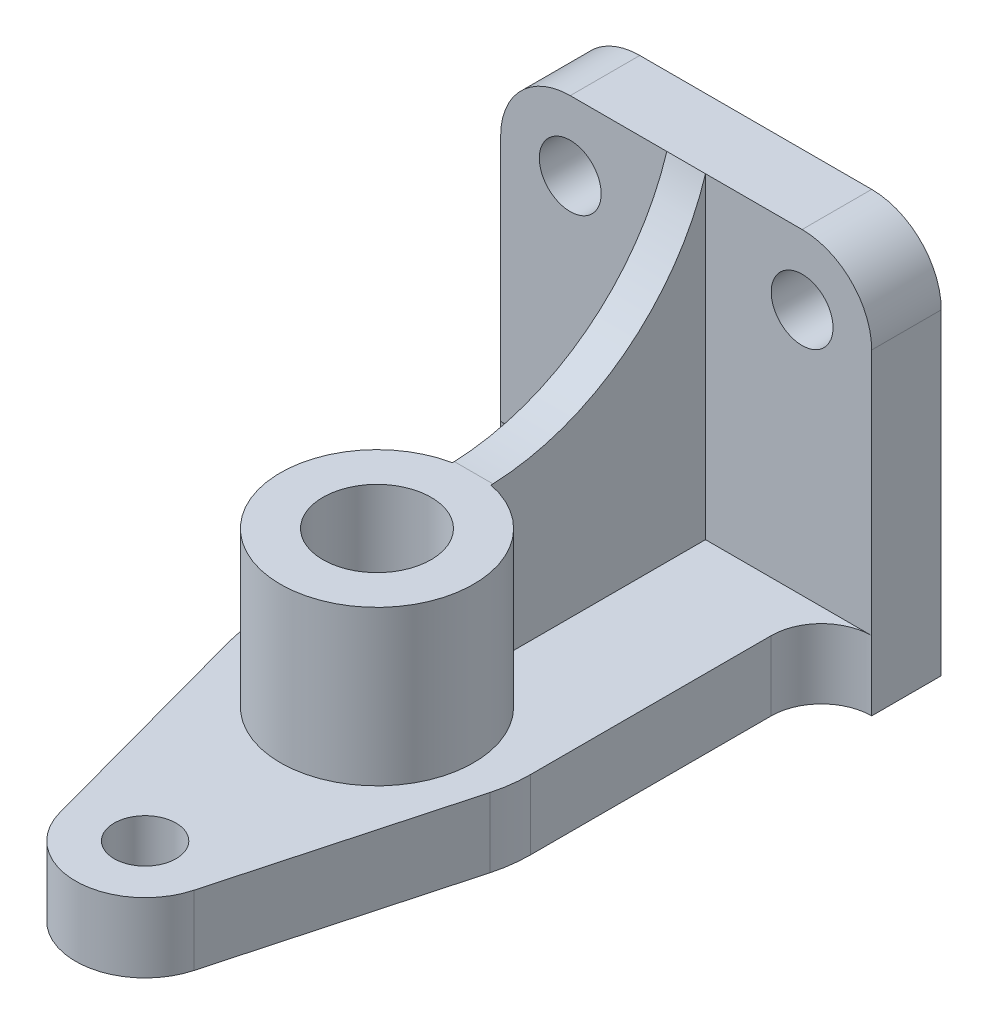
ISO-10303-21;
HEADER;
FILE_DESCRIPTION(('STEP AP214'),'2;1');
FILE_NAME('part.step','',(''),(''),'','','');
FILE_SCHEMA(('AUTOMOTIVE_DESIGN { 1 0 10303 214 1 1 1 1 }'));
ENDSEC;
DATA;
#1=APPLICATION_CONTEXT('core data for automotive mechanical design processes');
#2=APPLICATION_PROTOCOL_DEFINITION('international standard','automotive_design',2000,#1);
#3=PRODUCT_CONTEXT('',#1,'mechanical');
#4=PRODUCT('Part','Part','',(#3));
#5=PRODUCT_RELATED_PRODUCT_CATEGORY('part','',(#4));
#6=PRODUCT_DEFINITION_FORMATION('','',#4);
#7=PRODUCT_DEFINITION_CONTEXT('part definition',#1,'design');
#8=PRODUCT_DEFINITION('design','',#6,#7);
#9=PRODUCT_DEFINITION_SHAPE('','',#8);
#10=(LENGTH_UNIT() NAMED_UNIT(*) SI_UNIT(.MILLI.,.METRE.));
#11=(NAMED_UNIT(*) PLANE_ANGLE_UNIT() SI_UNIT($,.RADIAN.));
#12=(NAMED_UNIT(*) SI_UNIT($,.STERADIAN.) SOLID_ANGLE_UNIT());
#13=UNCERTAINTY_MEASURE_WITH_UNIT(LENGTH_MEASURE(1.E-05),#10,'distance_accuracy_value','');
#14=(GEOMETRIC_REPRESENTATION_CONTEXT(3) GLOBAL_UNCERTAINTY_ASSIGNED_CONTEXT((#13)) GLOBAL_UNIT_ASSIGNED_CONTEXT((#10,
#11,#12)) REPRESENTATION_CONTEXT('',''));
#15=CARTESIAN_POINT('',(0.,0.,0.));
#16=DIRECTION('',(0.,0.,1.));
#17=DIRECTION('',(1.,0.,0.));
#18=AXIS2_PLACEMENT_3D('',#15,#16,#17);
#19=CARTESIAN_POINT('',(18.,82.,18.));
#20=DIRECTION('',(0.,0.,-1.));
#21=DIRECTION('',(-1.,0.,0.));
#22=AXIS2_PLACEMENT_3D('',#19,#20,#21);
#23=PLANE('',#22);
#24=CARTESIAN_POINT('',(18.,82.,18.));
#25=DIRECTION('',(0.,0.,1.));
#26=DIRECTION('',(1.,0.,0.));
#27=AXIS2_PLACEMENT_3D('',#24,#25,#26);
#28=CIRCLE('',#27,8.);
#29=CARTESIAN_POINT('',(26.,82.,18.));
#30=VERTEX_POINT('',#29);
#31=EDGE_CURVE('E290',#30,#30,#28,.T.);
#32=ORIENTED_EDGE('',*,*,#31,.F.);
#33=EDGE_LOOP('',(#32));
#34=FACE_BOUND('',#33,.T.);
#35=DIRECTION('',(0.,-1.,0.));
#36=VECTOR('',#35,1.);
#37=CARTESIAN_POINT('',(43.,82.,18.));
#38=LINE('',#37,#36);
#39=CARTESIAN_POINT('',(43.,100.,18.));
#40=VERTEX_POINT('',#39);
#41=CARTESIAN_POINT('',(43.,18.,18.));
#42=VERTEX_POINT('',#41);
#43=EDGE_CURVE('E209',#40,#42,#38,.T.);
#44=ORIENTED_EDGE('',*,*,#43,.F.);
#45=DIRECTION('',(-1.,0.,0.));
#46=VECTOR('',#45,1.);
#47=CARTESIAN_POINT('',(18.0000000000001,100.,18.));
#48=LINE('',#47,#46);
#49=CARTESIAN_POINT('',(18.0000000000001,100.,18.));
#50=VERTEX_POINT('',#49);
#51=EDGE_CURVE('E303',#40,#50,#48,.T.);
#52=ORIENTED_EDGE('',*,*,#51,.T.);
#53=CARTESIAN_POINT('',(18.,82.,18.));
#54=DIRECTION('',(0.,0.,1.));
#55=DIRECTION('',(-1.,0.,0.));
#56=AXIS2_PLACEMENT_3D('',#53,#54,#55);
#57=CIRCLE('',#56,18.);
#58=CARTESIAN_POINT('',(0.,81.9999999999999,18.));
#59=VERTEX_POINT('',#58);
#60=EDGE_CURVE('E310',#50,#59,#57,.T.);
#61=ORIENTED_EDGE('',*,*,#60,.T.);
#62=DIRECTION('',(0.,-1.,0.));
#63=VECTOR('',#62,1.);
#64=CARTESIAN_POINT('',(0.,0.,18.));
#65=LINE('',#64,#63);
#66=CARTESIAN_POINT('',(0.,18.,18.));
#67=VERTEX_POINT('',#66);
#68=EDGE_CURVE('E291',#59,#67,#65,.T.);
#69=ORIENTED_EDGE('',*,*,#68,.T.);
#70=DIRECTION('',(1.,0.,0.));
#71=VECTOR('',#70,1.);
#72=CARTESIAN_POINT('',(13.,18.,18.));
#73=LINE('',#72,#71);
#74=EDGE_CURVE('E279',#67,#42,#73,.T.);
#75=ORIENTED_EDGE('',*,*,#74,.T.);
#76=EDGE_LOOP('',(#44,#52,#61,#69,#75));
#77=FACE_BOUND('',#76,.T.);
#78=ADVANCED_FACE('F45',(#34,#77),#23,.F.);
#79=CARTESIAN_POINT('',(0.,0.,18.));
#80=DIRECTION('',(0.,1.,0.));
#81=DIRECTION('',(0.,0.,1.));
#82=AXIS2_PLACEMENT_3D('',#79,#80,#81);
#83=PLANE('',#82);
#84=CARTESIAN_POINT('',(48.,0.,158.));
#85=DIRECTION('',(0.,1.,0.));
#86=DIRECTION('',(0.,0.,1.));
#87=AXIS2_PLACEMENT_3D('',#84,#85,#86);
#88=CIRCLE('',#87,8.);
#89=CARTESIAN_POINT('',(48.,0.,166.));
#90=VERTEX_POINT('',#89);
#91=EDGE_CURVE('E217',#90,#90,#88,.T.);
#92=ORIENTED_EDGE('',*,*,#91,.T.);
#93=EDGE_LOOP('',(#92));
#94=FACE_BOUND('',#93,.T.);
#95=DIRECTION('',(-0.262825333985644,0.,0.964843429689675));
#96=VECTOR('',#95,1.);
#97=CARTESIAN_POINT('',(97.5534197688363,0.,44.5737521168928));
#98=LINE('',#97,#96);
#99=CARTESIAN_POINT('',(81.7695200391386,0.,102.517146378541));
#100=VERTEX_POINT('',#99);
#101=CARTESIAN_POINT('',(65.3671817344141,0.,162.730856011742));
#102=VERTEX_POINT('',#101);
#103=EDGE_CURVE('E251',#100,#102,#98,.T.);
#104=ORIENTED_EDGE('',*,*,#103,.T.);
#105=CARTESIAN_POINT('',(48.,0.,158.));
#106=DIRECTION('',(0.,1.,0.));
#107=DIRECTION('',(0.,0.,1.));
#108=AXIS2_PLACEMENT_3D('',#105,#106,#107);
#109=CIRCLE('',#108,18.);
#110=CARTESIAN_POINT('',(30.6328182655859,0.,162.730856011742));
#111=VERTEX_POINT('',#110);
#112=EDGE_CURVE('E228',#111,#102,#109,.T.);
#113=ORIENTED_EDGE('',*,*,#112,.F.);
#114=DIRECTION('',(0.262825333985644,0.,0.964843429689675));
#115=VECTOR('',#114,1.);
#116=CARTESIAN_POINT('',(-8.18482676256409,0.,20.2295636382967));
#117=LINE('',#116,#115);
#118=CARTESIAN_POINT('',(14.2304799608614,0.,102.51714637854));
#119=VERTEX_POINT('',#118);
#120=EDGE_CURVE('E260',#119,#111,#117,.T.);
#121=ORIENTED_EDGE('',*,*,#120,.F.);
#122=CARTESIAN_POINT('',(48.,0.,93.3182596890428));
#123=DIRECTION('',(0.,1.,0.));
#124=DIRECTION('',(0.,0.,1.));
#125=AXIS2_PLACEMENT_3D('',#122,#123,#124);
#126=CIRCLE('',#125,35.);
#127=CARTESIAN_POINT('',(13.,0.,93.3182596890427));
#128=VERTEX_POINT('',#127);
#129=EDGE_CURVE('E255',#128,#119,#126,.T.);
#130=ORIENTED_EDGE('',*,*,#129,.F.);
#131=DIRECTION('',(0.,0.,-1.));
#132=VECTOR('',#131,1.);
#133=CARTESIAN_POINT('',(13.,0.,18.));
#134=LINE('',#133,#132);
#135=CARTESIAN_POINT('',(13.,0.,31.));
#136=VERTEX_POINT('',#135);
#137=EDGE_CURVE('E272',#128,#136,#134,.T.);
#138=ORIENTED_EDGE('',*,*,#137,.T.);
#139=CARTESIAN_POINT('',(0.,0.,31.));
#140=DIRECTION('',(0.,1.,0.));
#141=DIRECTION('',(0.,0.,1.));
#142=AXIS2_PLACEMENT_3D('',#139,#140,#141);
#143=CIRCLE('',#142,13.);
#144=CARTESIAN_POINT('',(0.,0.,18.));
#145=VERTEX_POINT('',#144);
#146=EDGE_CURVE('E346',#136,#145,#143,.T.);
#147=ORIENTED_EDGE('',*,*,#146,.T.);
#148=DIRECTION('',(0.,0.,-1.));
#149=VECTOR('',#148,1.);
#150=CARTESIAN_POINT('',(0.,0.,18.));
#151=LINE('',#150,#149);
#152=CARTESIAN_POINT('',(0.,0.,0.));
#153=VERTEX_POINT('',#152);
#154=EDGE_CURVE('E337',#145,#153,#151,.T.);
#155=ORIENTED_EDGE('',*,*,#154,.T.);
#156=DIRECTION('',(1.,0.,0.));
#157=VECTOR('',#156,1.);
#158=CARTESIAN_POINT('',(0.,0.,0.));
#159=LINE('',#158,#157);
#160=CARTESIAN_POINT('',(96.,0.,0.));
#161=VERTEX_POINT('',#160);
#162=EDGE_CURVE('E315',#153,#161,#159,.T.);
#163=ORIENTED_EDGE('',*,*,#162,.T.);
#164=DIRECTION('',(0.,0.,-1.));
#165=VECTOR('',#164,1.);
#166=CARTESIAN_POINT('',(96.,0.,18.));
#167=LINE('',#166,#165);
#168=CARTESIAN_POINT('',(96.,0.,18.));
#169=VERTEX_POINT('',#168);
#170=EDGE_CURVE('E331',#169,#161,#167,.T.);
#171=ORIENTED_EDGE('',*,*,#170,.F.);
#172=CARTESIAN_POINT('',(96.,0.,31.));
#173=DIRECTION('',(0.,1.,0.));
#174=DIRECTION('',(0.,0.,1.));
#175=AXIS2_PLACEMENT_3D('',#172,#173,#174);
#176=CIRCLE('',#175,13.);
#177=CARTESIAN_POINT('',(83.,0.,31.));
#178=VERTEX_POINT('',#177);
#179=EDGE_CURVE('E355',#169,#178,#176,.T.);
#180=ORIENTED_EDGE('',*,*,#179,.T.);
#181=DIRECTION('',(0.,0.,-1.));
#182=VECTOR('',#181,1.);
#183=CARTESIAN_POINT('',(83.,0.,18.));
#184=LINE('',#183,#182);
#185=CARTESIAN_POINT('',(83.,0.,93.318259689043));
#186=VERTEX_POINT('',#185);
#187=EDGE_CURVE('E275',#186,#178,#184,.T.);
#188=ORIENTED_EDGE('',*,*,#187,.F.);
#189=CARTESIAN_POINT('',(48.,0.,93.318259689043));
#190=DIRECTION('',(0.,1.,0.));
#191=DIRECTION('',(0.,0.,1.));
#192=AXIS2_PLACEMENT_3D('',#189,#190,#191);
#193=CIRCLE('',#192,35.);
#194=EDGE_CURVE('E242',#100,#186,#193,.T.);
#195=ORIENTED_EDGE('',*,*,#194,.F.);
#196=EDGE_LOOP('',(#104,#113,#121,#130,#138,#147,#155,#163,#171,#180,#188,#195));
#197=FACE_BOUND('',#196,.T.);
#198=ADVANCED_FACE('F417',(#94,#197),#83,.F.);
#199=CARTESIAN_POINT('',(13.,18.,18.));
#200=DIRECTION('',(0.,1.,0.));
#201=DIRECTION('',(0.,0.,1.));
#202=AXIS2_PLACEMENT_3D('',#199,#200,#201);
#203=PLANE('',#202);
#204=CARTESIAN_POINT('',(48.,18.,158.));
#205=DIRECTION('',(0.,1.,0.));
#206=DIRECTION('',(0.,0.,1.));
#207=AXIS2_PLACEMENT_3D('',#204,#205,#206);
#208=CIRCLE('',#207,8.);
#209=CARTESIAN_POINT('',(48.,18.,166.));
#210=VERTEX_POINT('',#209);
#211=EDGE_CURVE('E218',#210,#210,#208,.T.);
#212=ORIENTED_EDGE('',*,*,#211,.F.);
#213=EDGE_LOOP('',(#212));
#214=FACE_BOUND('',#213,.T.);
#215=CARTESIAN_POINT('',(48.,18.,158.));
#216=DIRECTION('',(0.,1.,0.));
#217=DIRECTION('',(0.,0.,1.));
#218=AXIS2_PLACEMENT_3D('',#215,#216,#217);
#219=CIRCLE('',#218,18.);
#220=CARTESIAN_POINT('',(30.6328182655859,18.,162.730856011742));
#221=VERTEX_POINT('',#220);
#222=CARTESIAN_POINT('',(65.3671817344141,18.,162.730856011742));
#223=VERTEX_POINT('',#222);
#224=EDGE_CURVE('E221',#221,#223,#219,.T.);
#225=ORIENTED_EDGE('',*,*,#224,.T.);
#226=DIRECTION('',(-0.262825333985644,0.,0.964843429689675));
#227=VECTOR('',#226,1.);
#228=CARTESIAN_POINT('',(102.117955108573,18.,27.8171409282168));
#229=LINE('',#228,#227);
#230=CARTESIAN_POINT('',(81.7695200391386,18.,102.517146378541));
#231=VERTEX_POINT('',#230);
#232=EDGE_CURVE('E250',#231,#223,#229,.T.);
#233=ORIENTED_EDGE('',*,*,#232,.F.);
#234=CARTESIAN_POINT('',(48.,18.,93.318259689043));
#235=DIRECTION('',(0.,1.,0.));
#236=DIRECTION('',(0.,0.,1.));
#237=AXIS2_PLACEMENT_3D('',#234,#235,#236);
#238=CIRCLE('',#237,35.);
#239=CARTESIAN_POINT('',(83.,18.,93.3182596890429));
#240=VERTEX_POINT('',#239);
#241=EDGE_CURVE('E231',#231,#240,#238,.T.);
#242=ORIENTED_EDGE('',*,*,#241,.T.);
#243=DIRECTION('',(0.,0.,1.));
#244=VECTOR('',#243,1.);
#245=CARTESIAN_POINT('',(83.,18.,18.));
#246=LINE('',#245,#244);
#247=CARTESIAN_POINT('',(83.,18.,31.));
#248=VERTEX_POINT('',#247);
#249=EDGE_CURVE('E262',#248,#240,#246,.T.);
#250=ORIENTED_EDGE('',*,*,#249,.F.);
#251=CARTESIAN_POINT('',(96.,18.,31.));
#252=DIRECTION('',(0.,1.,0.));
#253=DIRECTION('',(0.,0.,1.));
#254=AXIS2_PLACEMENT_3D('',#251,#252,#253);
#255=CIRCLE('',#254,13.);
#256=CARTESIAN_POINT('',(96.,18.,18.));
#257=VERTEX_POINT('',#256);
#258=EDGE_CURVE('E348',#248,#257,#255,.F.);
#259=ORIENTED_EDGE('',*,*,#258,.T.);
#260=CARTESIAN_POINT('',(53.,18.,18.));
#261=VERTEX_POINT('',#260);
#262=EDGE_CURVE('E274',#261,#257,#73,.T.);
#263=ORIENTED_EDGE('',*,*,#262,.F.);
#264=DIRECTION('',(0.,0.,-1.));
#265=VECTOR('',#264,1.);
#266=CARTESIAN_POINT('',(53.,18.,18.));
#267=LINE('',#266,#265);
#268=CARTESIAN_POINT('',(53.,18.,73.5051025721682));
#269=VERTEX_POINT('',#268);
#270=EDGE_CURVE('E60',#269,#261,#267,.T.);
#271=ORIENTED_EDGE('',*,*,#270,.F.);
#272=CARTESIAN_POINT('',(48.,18.,98.));
#273=DIRECTION('',(0.,1.,0.));
#274=DIRECTION('',(0.,0.,1.));
#275=AXIS2_PLACEMENT_3D('',#272,#273,#274);
#276=CIRCLE('',#275,25.);
#277=CARTESIAN_POINT('',(43.,18.,73.5051025721682));
#278=VERTEX_POINT('',#277);
#279=EDGE_CURVE('E256',#278,#269,#276,.T.);
#280=ORIENTED_EDGE('',*,*,#279,.F.);
#281=DIRECTION('',(0.,0.,-1.));
#282=VECTOR('',#281,1.);
#283=CARTESIAN_POINT('',(43.,18.,18.));
#284=LINE('',#283,#282);
#285=EDGE_CURVE('E63',#278,#42,#284,.T.);
#286=ORIENTED_EDGE('',*,*,#285,.T.);
#287=ORIENTED_EDGE('',*,*,#74,.F.);
#288=CARTESIAN_POINT('',(0.,18.,31.));
#289=DIRECTION('',(0.,1.,0.));
#290=DIRECTION('',(0.,0.,1.));
#291=AXIS2_PLACEMENT_3D('',#288,#289,#290);
#292=CIRCLE('',#291,13.);
#293=CARTESIAN_POINT('',(13.,18.,31.));
#294=VERTEX_POINT('',#293);
#295=EDGE_CURVE('E343',#67,#294,#292,.F.);
#296=ORIENTED_EDGE('',*,*,#295,.T.);
#297=DIRECTION('',(0.,0.,1.));
#298=VECTOR('',#297,1.);
#299=CARTESIAN_POINT('',(13.,18.,18.));
#300=LINE('',#299,#298);
#301=CARTESIAN_POINT('',(13.,18.,93.3182596890427));
#302=VERTEX_POINT('',#301);
#303=EDGE_CURVE('E266',#294,#302,#300,.T.);
#304=ORIENTED_EDGE('',*,*,#303,.T.);
#305=CARTESIAN_POINT('',(48.,18.,93.3182596890428));
#306=DIRECTION('',(0.,1.,0.));
#307=DIRECTION('',(0.,0.,1.));
#308=AXIS2_PLACEMENT_3D('',#305,#306,#307);
#309=CIRCLE('',#308,35.);
#310=CARTESIAN_POINT('',(14.2304799608614,18.,102.51714637854));
#311=VERTEX_POINT('',#310);
#312=EDGE_CURVE('E236',#302,#311,#309,.T.);
#313=ORIENTED_EDGE('',*,*,#312,.T.);
#314=DIRECTION('',(0.262825333985644,0.,0.964843429689675));
#315=VECTOR('',#314,1.);
#316=CARTESIAN_POINT('',(-12.7493621023009,18.,3.47295244962065));
#317=LINE('',#316,#315);
#318=EDGE_CURVE('E237',#311,#221,#317,.T.);
#319=ORIENTED_EDGE('',*,*,#318,.T.);
#320=EDGE_LOOP('',(#225,#233,#242,#250,#259,#263,#271,#280,#286,#287,#296,#304,#313,#319));
#321=FACE_BOUND('',#320,.T.);
#322=ADVANCED_FACE('F370',(#214,#321),#203,.T.);
#323=CARTESIAN_POINT('',(78.,82.,18.));
#324=DIRECTION('',(0.,0.,1.));
#325=DIRECTION('',(1.,0.,0.));
#326=AXIS2_PLACEMENT_3D('',#323,#324,#325);
#327=CIRCLE('',#326,8.00000000000001);
#328=CARTESIAN_POINT('',(86.,82.,18.));
#329=VERTEX_POINT('',#328);
#330=EDGE_CURVE('E284',#329,#329,#327,.T.);
#331=ORIENTED_EDGE('',*,*,#330,.F.);
#332=EDGE_LOOP('',(#331));
#333=FACE_BOUND('',#332,.T.);
#334=CARTESIAN_POINT('',(77.9999999999999,100.,18.));
#335=VERTEX_POINT('',#334);
#336=CARTESIAN_POINT('',(53.,100.,18.));
#337=VERTEX_POINT('',#336);
#338=EDGE_CURVE('E302',#335,#337,#48,.T.);
#339=ORIENTED_EDGE('',*,*,#338,.T.);
#340=DIRECTION('',(0.,-1.,0.));
#341=VECTOR('',#340,1.);
#342=CARTESIAN_POINT('',(53.,82.,18.));
#343=LINE('',#342,#341);
#344=EDGE_CURVE('E211',#337,#261,#343,.T.);
#345=ORIENTED_EDGE('',*,*,#344,.T.);
#346=ORIENTED_EDGE('',*,*,#262,.T.);
#347=DIRECTION('',(0.,1.,0.));
#348=VECTOR('',#347,1.);
#349=CARTESIAN_POINT('',(96.,0.,18.));
#350=LINE('',#349,#348);
#351=CARTESIAN_POINT('',(96.,81.9999999999999,18.));
#352=VERTEX_POINT('',#351);
#353=EDGE_CURVE('E298',#257,#352,#350,.T.);
#354=ORIENTED_EDGE('',*,*,#353,.T.);
#355=CARTESIAN_POINT('',(78.,82.,18.));
#356=DIRECTION('',(0.,0.,1.));
#357=DIRECTION('',(-1.,0.,0.));
#358=AXIS2_PLACEMENT_3D('',#355,#356,#357);
#359=CIRCLE('',#358,18.);
#360=EDGE_CURVE('E301',#352,#335,#359,.T.);
#361=ORIENTED_EDGE('',*,*,#360,.T.);
#362=EDGE_LOOP('',(#339,#345,#346,#354,#361));
#363=FACE_BOUND('',#362,.T.);
#364=ADVANCED_FACE('F379',(#333,#363),#23,.F.);
#365=CARTESIAN_POINT('',(18.,82.,0.));
#366=DIRECTION('',(0.,0.,-1.));
#367=DIRECTION('',(-1.,0.,0.));
#368=AXIS2_PLACEMENT_3D('',#365,#366,#367);
#369=PLANE('',#368);
#370=DIRECTION('',(0.,1.,0.));
#371=VECTOR('',#370,1.);
#372=CARTESIAN_POINT('',(96.,0.,0.));
#373=LINE('',#372,#371);
#374=CARTESIAN_POINT('',(96.,81.9999999999999,0.));
#375=VERTEX_POINT('',#374);
#376=EDGE_CURVE('E313',#161,#375,#373,.T.);
#377=ORIENTED_EDGE('',*,*,#376,.F.);
#378=ORIENTED_EDGE('',*,*,#162,.F.);
#379=DIRECTION('',(0.,-1.,0.));
#380=VECTOR('',#379,1.);
#381=CARTESIAN_POINT('',(0.,0.,0.));
#382=LINE('',#381,#380);
#383=CARTESIAN_POINT('',(0.,81.9999999999999,0.));
#384=VERTEX_POINT('',#383);
#385=EDGE_CURVE('E287',#384,#153,#382,.T.);
#386=ORIENTED_EDGE('',*,*,#385,.F.);
#387=CARTESIAN_POINT('',(18.,82.,0.));
#388=DIRECTION('',(0.,0.,1.));
#389=DIRECTION('',(-1.,0.,0.));
#390=AXIS2_PLACEMENT_3D('',#387,#388,#389);
#391=CIRCLE('',#390,18.);
#392=CARTESIAN_POINT('',(18.0000000000001,100.,0.));
#393=VERTEX_POINT('',#392);
#394=EDGE_CURVE('E318',#393,#384,#391,.T.);
#395=ORIENTED_EDGE('',*,*,#394,.F.);
#396=DIRECTION('',(-1.,0.,0.));
#397=VECTOR('',#396,1.);
#398=CARTESIAN_POINT('',(18.0000000000001,100.,0.));
#399=LINE('',#398,#397);
#400=CARTESIAN_POINT('',(77.9999999999999,100.,0.));
#401=VERTEX_POINT('',#400);
#402=EDGE_CURVE('E319',#401,#393,#399,.T.);
#403=ORIENTED_EDGE('',*,*,#402,.F.);
#404=CARTESIAN_POINT('',(78.,82.,0.));
#405=DIRECTION('',(0.,0.,1.));
#406=DIRECTION('',(-1.,0.,0.));
#407=AXIS2_PLACEMENT_3D('',#404,#405,#406);
#408=CIRCLE('',#407,18.);
#409=EDGE_CURVE('E317',#375,#401,#408,.T.);
#410=ORIENTED_EDGE('',*,*,#409,.F.);
#411=EDGE_LOOP('',(#377,#378,#386,#395,#403,#410));
#412=FACE_BOUND('',#411,.T.);
#413=CARTESIAN_POINT('',(78.,82.,0.));
#414=DIRECTION('',(0.,0.,1.));
#415=DIRECTION('',(1.,0.,0.));
#416=AXIS2_PLACEMENT_3D('',#413,#414,#415);
#417=CIRCLE('',#416,8.00000000000001);
#418=CARTESIAN_POINT('',(86.,82.,0.));
#419=VERTEX_POINT('',#418);
#420=EDGE_CURVE('E278',#419,#419,#417,.T.);
#421=ORIENTED_EDGE('',*,*,#420,.T.);
#422=EDGE_LOOP('',(#421));
#423=FACE_BOUND('',#422,.T.);
#424=CARTESIAN_POINT('',(18.,82.,0.));
#425=DIRECTION('',(0.,0.,1.));
#426=DIRECTION('',(1.,0.,0.));
#427=AXIS2_PLACEMENT_3D('',#424,#425,#426);
#428=CIRCLE('',#427,8.);
#429=CARTESIAN_POINT('',(26.,82.,0.));
#430=VERTEX_POINT('',#429);
#431=EDGE_CURVE('E283',#430,#430,#428,.T.);
#432=ORIENTED_EDGE('',*,*,#431,.T.);
#433=EDGE_LOOP('',(#432));
#434=FACE_BOUND('',#433,.T.);
#435=ADVANCED_FACE('F434',(#412,#423,#434),#369,.T.);
#436=CARTESIAN_POINT('',(0.,0.,18.));
#437=DIRECTION('',(1.,0.,0.));
#438=DIRECTION('',(0.,0.,-1.));
#439=AXIS2_PLACEMENT_3D('',#436,#437,#438);
#440=PLANE('',#439);
#441=ORIENTED_EDGE('',*,*,#385,.T.);
#442=ORIENTED_EDGE('',*,*,#154,.F.);
#443=EDGE_CURVE('E300',#67,#145,#65,.T.);
#444=ORIENTED_EDGE('',*,*,#443,.F.);
#445=ORIENTED_EDGE('',*,*,#68,.F.);
#446=DIRECTION('',(0.,0.,-1.));
#447=VECTOR('',#446,1.);
#448=CARTESIAN_POINT('',(0.,81.9999999999999,18.));
#449=LINE('',#448,#447);
#450=EDGE_CURVE('E307',#59,#384,#449,.T.);
#451=ORIENTED_EDGE('',*,*,#450,.T.);
#452=EDGE_LOOP('',(#441,#442,#444,#445,#451));
#453=FACE_BOUND('',#452,.T.);
#454=ADVANCED_FACE('F402',(#453),#440,.F.);
#455=CARTESIAN_POINT('',(96.,0.,18.));
#456=DIRECTION('',(-1.,0.,0.));
#457=DIRECTION('',(0.,0.,1.));
#458=AXIS2_PLACEMENT_3D('',#455,#456,#457);
#459=PLANE('',#458);
#460=ORIENTED_EDGE('',*,*,#376,.T.);
#461=DIRECTION('',(0.,0.,-1.));
#462=VECTOR('',#461,1.);
#463=CARTESIAN_POINT('',(96.,81.9999999999999,18.));
#464=LINE('',#463,#462);
#465=EDGE_CURVE('E327',#352,#375,#464,.T.);
#466=ORIENTED_EDGE('',*,*,#465,.F.);
#467=ORIENTED_EDGE('',*,*,#353,.F.);
#468=EDGE_CURVE('E296',#169,#257,#350,.T.);
#469=ORIENTED_EDGE('',*,*,#468,.F.);
#470=ORIENTED_EDGE('',*,*,#170,.T.);
#471=EDGE_LOOP('',(#460,#466,#467,#469,#470));
#472=FACE_BOUND('',#471,.T.);
#473=ADVANCED_FACE('F380',(#472),#459,.F.);
#474=CARTESIAN_POINT('',(78.,82.,18.));
#475=DIRECTION('',(0.,0.,-1.));
#476=DIRECTION('',(-1.,0.,0.));
#477=AXIS2_PLACEMENT_3D('',#474,#475,#476);
#478=CYLINDRICAL_SURFACE('',#477,18.);
#479=ORIENTED_EDGE('',*,*,#409,.T.);
#480=DIRECTION('',(0.,0.,-1.));
#481=VECTOR('',#480,1.);
#482=CARTESIAN_POINT('',(77.9999999999999,100.,18.));
#483=LINE('',#482,#481);
#484=EDGE_CURVE('E326',#335,#401,#483,.T.);
#485=ORIENTED_EDGE('',*,*,#484,.F.);
#486=ORIENTED_EDGE('',*,*,#360,.F.);
#487=ORIENTED_EDGE('',*,*,#465,.T.);
#488=EDGE_LOOP('',(#479,#485,#486,#487));
#489=FACE_BOUND('',#488,.T.);
#490=ADVANCED_FACE('F438',(#489),#478,.T.);
#491=CARTESIAN_POINT('',(18.0000000000001,100.,18.));
#492=DIRECTION('',(0.,-1.,0.));
#493=DIRECTION('',(0.,0.,-1.));
#494=AXIS2_PLACEMENT_3D('',#491,#492,#493);
#495=PLANE('',#494);
#496=ORIENTED_EDGE('',*,*,#402,.T.);
#497=DIRECTION('',(0.,0.,-1.));
#498=VECTOR('',#497,1.);
#499=CARTESIAN_POINT('',(18.0000000000001,100.,18.));
#500=LINE('',#499,#498);
#501=EDGE_CURVE('E321',#50,#393,#500,.T.);
#502=ORIENTED_EDGE('',*,*,#501,.F.);
#503=ORIENTED_EDGE('',*,*,#51,.F.);
#504=DIRECTION('',(1.,0.,0.));
#505=VECTOR('',#504,1.);
#506=CARTESIAN_POINT('',(48.,100.,18.));
#507=LINE('',#506,#505);
#508=EDGE_CURVE('E194',#40,#337,#507,.T.);
#509=ORIENTED_EDGE('',*,*,#508,.T.);
#510=ORIENTED_EDGE('',*,*,#338,.F.);
#511=ORIENTED_EDGE('',*,*,#484,.T.);
#512=EDGE_LOOP('',(#496,#502,#503,#509,#510,#511));
#513=FACE_BOUND('',#512,.T.);
#514=ADVANCED_FACE('F394',(#513),#495,.F.);
#515=CARTESIAN_POINT('',(18.,82.,18.));
#516=DIRECTION('',(0.,0.,-1.));
#517=DIRECTION('',(-1.,0.,0.));
#518=AXIS2_PLACEMENT_3D('',#515,#516,#517);
#519=CYLINDRICAL_SURFACE('',#518,18.);
#520=ORIENTED_EDGE('',*,*,#394,.T.);
#521=ORIENTED_EDGE('',*,*,#450,.F.);
#522=ORIENTED_EDGE('',*,*,#60,.F.);
#523=ORIENTED_EDGE('',*,*,#501,.T.);
#524=EDGE_LOOP('',(#520,#521,#522,#523));
#525=FACE_BOUND('',#524,.T.);
#526=ADVANCED_FACE('F400',(#525),#519,.T.);
#527=CARTESIAN_POINT('',(18.,82.,18.));
#528=DIRECTION('',(0.,0.,-1.));
#529=DIRECTION('',(-1.,0.,0.));
#530=AXIS2_PLACEMENT_3D('',#527,#528,#529);
#531=CYLINDRICAL_SURFACE('',#530,8.);
#532=ORIENTED_EDGE('',*,*,#31,.T.);
#533=EDGE_LOOP('',(#532));
#534=FACE_BOUND('',#533,.T.);
#535=ORIENTED_EDGE('',*,*,#431,.F.);
#536=EDGE_LOOP('',(#535));
#537=FACE_BOUND('',#536,.T.);
#538=ADVANCED_FACE('F471',(#534,#537),#531,.F.);
#539=CARTESIAN_POINT('',(78.,82.,18.));
#540=DIRECTION('',(0.,0.,-1.));
#541=DIRECTION('',(-1.,0.,0.));
#542=AXIS2_PLACEMENT_3D('',#539,#540,#541);
#543=CYLINDRICAL_SURFACE('',#542,8.00000000000001);
#544=ORIENTED_EDGE('',*,*,#330,.T.);
#545=EDGE_LOOP('',(#544));
#546=FACE_BOUND('',#545,.T.);
#547=ORIENTED_EDGE('',*,*,#420,.F.);
#548=EDGE_LOOP('',(#547));
#549=FACE_BOUND('',#548,.T.);
#550=ADVANCED_FACE('F472',(#546,#549),#543,.F.);
#551=CARTESIAN_POINT('',(13.,0.,0.));
#552=DIRECTION('',(1.,0.,0.));
#553=DIRECTION('',(0.,0.,-1.));
#554=AXIS2_PLACEMENT_3D('',#551,#552,#553);
#555=PLANE('',#554);
#556=ORIENTED_EDGE('',*,*,#137,.F.);
#557=DIRECTION('',(0.,1.,0.));
#558=VECTOR('',#557,1.);
#559=CARTESIAN_POINT('',(13.,-22.,93.3182596890428));
#560=LINE('',#559,#558);
#561=EDGE_CURVE('E12',#128,#302,#560,.T.);
#562=ORIENTED_EDGE('',*,*,#561,.T.);
#563=ORIENTED_EDGE('',*,*,#303,.F.);
#564=DIRECTION('',(0.,1.,0.));
#565=VECTOR('',#564,1.);
#566=CARTESIAN_POINT('',(13.,0.,31.));
#567=LINE('',#566,#565);
#568=EDGE_CURVE('E339',#294,#136,#567,.F.);
#569=ORIENTED_EDGE('',*,*,#568,.T.);
#570=EDGE_LOOP('',(#556,#562,#563,#569));
#571=FACE_BOUND('',#570,.T.);
#572=ADVANCED_FACE('F415',(#571),#555,.F.);
#573=CARTESIAN_POINT('',(83.,0.,0.));
#574=DIRECTION('',(1.,0.,0.));
#575=DIRECTION('',(0.,0.,-1.));
#576=AXIS2_PLACEMENT_3D('',#573,#574,#575);
#577=PLANE('',#576);
#578=DIRECTION('',(0.,1.,0.));
#579=VECTOR('',#578,1.);
#580=CARTESIAN_POINT('',(83.,-22.,93.318259689043));
#581=LINE('',#580,#579);
#582=EDGE_CURVE('E49',#186,#240,#581,.T.);
#583=ORIENTED_EDGE('',*,*,#582,.F.);
#584=ORIENTED_EDGE('',*,*,#187,.T.);
#585=DIRECTION('',(0.,1.,0.));
#586=VECTOR('',#585,1.);
#587=CARTESIAN_POINT('',(83.,0.,31.));
#588=LINE('',#587,#586);
#589=EDGE_CURVE('E345',#178,#248,#588,.T.);
#590=ORIENTED_EDGE('',*,*,#589,.T.);
#591=ORIENTED_EDGE('',*,*,#249,.T.);
#592=EDGE_LOOP('',(#583,#584,#590,#591));
#593=FACE_BOUND('',#592,.T.);
#594=ADVANCED_FACE('F368',(#593),#577,.T.);
#595=CARTESIAN_POINT('',(0.,82.,31.));
#596=DIRECTION('',(0.,-1.,0.));
#597=DIRECTION('',(0.,0.,-1.));
#598=AXIS2_PLACEMENT_3D('',#595,#596,#597);
#599=CYLINDRICAL_SURFACE('',#598,13.);
#600=ORIENTED_EDGE('',*,*,#146,.F.);
#601=ORIENTED_EDGE('',*,*,#568,.F.);
#602=ORIENTED_EDGE('',*,*,#295,.F.);
#603=ORIENTED_EDGE('',*,*,#443,.T.);
#604=EDGE_LOOP('',(#600,#601,#602,#603));
#605=FACE_BOUND('',#604,.T.);
#606=ADVANCED_FACE('F409',(#605),#599,.F.);
#607=CARTESIAN_POINT('',(96.,0.,31.));
#608=DIRECTION('',(0.,1.,0.));
#609=DIRECTION('',(0.,0.,1.));
#610=AXIS2_PLACEMENT_3D('',#607,#608,#609);
#611=CYLINDRICAL_SURFACE('',#610,13.);
#612=ORIENTED_EDGE('',*,*,#179,.F.);
#613=ORIENTED_EDGE('',*,*,#468,.T.);
#614=ORIENTED_EDGE('',*,*,#258,.F.);
#615=ORIENTED_EDGE('',*,*,#589,.F.);
#616=EDGE_LOOP('',(#612,#613,#614,#615));
#617=FACE_BOUND('',#616,.T.);
#618=ADVANCED_FACE('F42',(#617),#611,.F.);
#619=CARTESIAN_POINT('',(48.,58.,98.));
#620=DIRECTION('',(0.,-1.,0.));
#621=DIRECTION('',(0.,0.,-1.));
#622=AXIS2_PLACEMENT_3D('',#619,#620,#621);
#623=CYLINDRICAL_SURFACE('',#622,14.);
#624=CARTESIAN_POINT('',(48.,18.,98.));
#625=DIRECTION('',(0.,1.,0.));
#626=DIRECTION('',(0.,0.,1.));
#627=AXIS2_PLACEMENT_3D('',#624,#625,#626);
#628=CIRCLE('',#627,14.);
#629=CARTESIAN_POINT('',(48.,18.,112.));
#630=VERTEX_POINT('',#629);
#631=EDGE_CURVE('E352',#630,#630,#628,.F.);
#632=ORIENTED_EDGE('',*,*,#631,.T.);
#633=EDGE_LOOP('',(#632));
#634=FACE_BOUND('',#633,.T.);
#635=CARTESIAN_POINT('',(48.,58.,98.));
#636=DIRECTION('',(0.,1.,0.));
#637=DIRECTION('',(0.,0.,1.));
#638=AXIS2_PLACEMENT_3D('',#635,#636,#637);
#639=CIRCLE('',#638,14.);
#640=CARTESIAN_POINT('',(48.,58.,112.));
#641=VERTEX_POINT('',#640);
#642=EDGE_CURVE('E258',#641,#641,#639,.T.);
#643=ORIENTED_EDGE('',*,*,#642,.T.);
#644=EDGE_LOOP('',(#643));
#645=FACE_BOUND('',#644,.T.);
#646=ADVANCED_FACE('F489',(#634,#645),#623,.F.);
#647=CARTESIAN_POINT('',(48.,58.,98.));
#648=DIRECTION('',(0.,-1.,0.));
#649=DIRECTION('',(0.,0.,-1.));
#650=AXIS2_PLACEMENT_3D('',#647,#648,#649);
#651=CYLINDRICAL_SURFACE('',#650,25.);
#652=DIRECTION('',(0.,-1.,0.));
#653=VECTOR('',#652,1.);
#654=CARTESIAN_POINT('',(53.,58.,73.5051025721682));
#655=LINE('',#654,#653);
#656=CARTESIAN_POINT('',(53.,58.,73.5051025721682));
#657=VERTEX_POINT('',#656);
#658=EDGE_CURVE('E219',#269,#657,#655,.F.);
#659=ORIENTED_EDGE('',*,*,#658,.T.);
#660=CARTESIAN_POINT('',(48.,58.,98.));
#661=DIRECTION('',(0.,1.,0.));
#662=DIRECTION('',(0.,0.,1.));
#663=AXIS2_PLACEMENT_3D('',#660,#661,#662);
#664=CIRCLE('',#663,25.);
#665=CARTESIAN_POINT('',(43.,58.,73.5051025721682));
#666=VERTEX_POINT('',#665);
#667=EDGE_CURVE('E265',#666,#657,#664,.T.);
#668=ORIENTED_EDGE('',*,*,#667,.F.);
#669=DIRECTION('',(0.,-1.,0.));
#670=VECTOR('',#669,1.);
#671=CARTESIAN_POINT('',(43.,58.,73.5051025721682));
#672=LINE('',#671,#670);
#673=EDGE_CURVE('E205',#278,#666,#672,.F.);
#674=ORIENTED_EDGE('',*,*,#673,.F.);
#675=ORIENTED_EDGE('',*,*,#279,.T.);
#676=EDGE_LOOP('',(#659,#668,#674,#675));
#677=FACE_BOUND('',#676,.T.);
#678=ADVANCED_FACE('F387',(#677),#651,.T.);
#679=CARTESIAN_POINT('',(0.,58.,0.));
#680=DIRECTION('',(0.,1.,0.));
#681=DIRECTION('',(0.,0.,1.));
#682=AXIS2_PLACEMENT_3D('',#679,#680,#681);
#683=PLANE('',#682);
#684=ORIENTED_EDGE('',*,*,#667,.T.);
#685=DIRECTION('',(0.,0.,-1.));
#686=VECTOR('',#685,1.);
#687=CARTESIAN_POINT('',(53.,58.,74.3832226340811));
#688=LINE('',#687,#686);
#689=CARTESIAN_POINT('',(53.,58.,73.));
#690=VERTEX_POINT('',#689);
#691=EDGE_CURVE('E189',#657,#690,#688,.T.);
#692=ORIENTED_EDGE('',*,*,#691,.T.);
#693=DIRECTION('',(1.,0.,0.));
#694=VECTOR('',#693,1.);
#695=CARTESIAN_POINT('',(48.,58.,73.));
#696=LINE('',#695,#694);
#697=CARTESIAN_POINT('',(43.,58.,73.));
#698=VERTEX_POINT('',#697);
#699=EDGE_CURVE('E179',#698,#690,#696,.T.);
#700=ORIENTED_EDGE('',*,*,#699,.F.);
#701=DIRECTION('',(0.,0.,1.));
#702=VECTOR('',#701,1.);
#703=CARTESIAN_POINT('',(43.,58.,73.));
#704=LINE('',#703,#702);
#705=EDGE_CURVE('E184',#698,#666,#704,.T.);
#706=ORIENTED_EDGE('',*,*,#705,.T.);
#707=EDGE_LOOP('',(#684,#692,#700,#706));
#708=FACE_BOUND('',#707,.T.);
#709=ORIENTED_EDGE('',*,*,#642,.F.);
#710=EDGE_LOOP('',(#709));
#711=FACE_BOUND('',#710,.T.);
#712=ADVANCED_FACE('F182',(#708,#711),#683,.T.);
#713=ORIENTED_EDGE('',*,*,#631,.F.);
#714=EDGE_LOOP('',(#713));
#715=FACE_BOUND('',#714,.T.);
#716=ADVANCED_FACE('F466',(#715),#203,.T.);
#717=CARTESIAN_POINT('',(102.117955108573,-22.,27.8171409282168));
#718=DIRECTION('',(-0.964843429689675,0.,-0.262825333985644));
#719=DIRECTION('',(-0.262825333985644,0.,0.964843429689675));
#720=AXIS2_PLACEMENT_3D('',#717,#718,#719);
#721=PLANE('',#720);
#722=DIRECTION('',(0.,1.,0.));
#723=VECTOR('',#722,1.);
#724=CARTESIAN_POINT('',(81.7695200391386,-22.,102.517146378541));
#725=LINE('',#724,#723);
#726=EDGE_CURVE('E239',#100,#231,#725,.T.);
#727=ORIENTED_EDGE('',*,*,#726,.T.);
#728=ORIENTED_EDGE('',*,*,#232,.T.);
#729=DIRECTION('',(0.,1.,0.));
#730=VECTOR('',#729,1.);
#731=CARTESIAN_POINT('',(65.3671817344141,0.,162.730856011742));
#732=LINE('',#731,#730);
#733=EDGE_CURVE('E229',#102,#223,#732,.T.);
#734=ORIENTED_EDGE('',*,*,#733,.F.);
#735=ORIENTED_EDGE('',*,*,#103,.F.);
#736=EDGE_LOOP('',(#727,#728,#734,#735));
#737=FACE_BOUND('',#736,.T.);
#738=ADVANCED_FACE('F431',(#737),#721,.F.);
#739=CARTESIAN_POINT('',(48.,-22.,93.318259689043));
#740=DIRECTION('',(0.,1.,0.));
#741=DIRECTION('',(0.,0.,1.));
#742=AXIS2_PLACEMENT_3D('',#739,#740,#741);
#743=CYLINDRICAL_SURFACE('',#742,35.);
#744=ORIENTED_EDGE('',*,*,#194,.T.);
#745=ORIENTED_EDGE('',*,*,#582,.T.);
#746=ORIENTED_EDGE('',*,*,#241,.F.);
#747=ORIENTED_EDGE('',*,*,#726,.F.);
#748=EDGE_LOOP('',(#744,#745,#746,#747));
#749=FACE_BOUND('',#748,.T.);
#750=ADVANCED_FACE('F359',(#749),#743,.T.);
#751=CARTESIAN_POINT('',(-12.7493621023009,-22.,3.47295244962064));
#752=DIRECTION('',(-0.964843429689675,0.,0.262825333985644));
#753=DIRECTION('',(0.262825333985644,0.,0.964843429689675));
#754=AXIS2_PLACEMENT_3D('',#751,#752,#753);
#755=PLANE('',#754);
#756=ORIENTED_EDGE('',*,*,#120,.T.);
#757=DIRECTION('',(0.,1.,0.));
#758=VECTOR('',#757,1.);
#759=CARTESIAN_POINT('',(30.6328182655859,0.,162.730856011742));
#760=LINE('',#759,#758);
#761=EDGE_CURVE('E226',#111,#221,#760,.T.);
#762=ORIENTED_EDGE('',*,*,#761,.T.);
#763=ORIENTED_EDGE('',*,*,#318,.F.);
#764=DIRECTION('',(0.,1.,0.));
#765=VECTOR('',#764,1.);
#766=CARTESIAN_POINT('',(14.2304799608614,-22.,102.51714637854));
#767=LINE('',#766,#765);
#768=EDGE_CURVE('E245',#119,#311,#767,.T.);
#769=ORIENTED_EDGE('',*,*,#768,.F.);
#770=EDGE_LOOP('',(#756,#762,#763,#769));
#771=FACE_BOUND('',#770,.T.);
#772=ADVANCED_FACE('F425',(#771),#755,.T.);
#773=CARTESIAN_POINT('',(48.,-22.,93.3182596890428));
#774=DIRECTION('',(0.,1.,0.));
#775=DIRECTION('',(0.,0.,1.));
#776=AXIS2_PLACEMENT_3D('',#773,#774,#775);
#777=CYLINDRICAL_SURFACE('',#776,35.);
#778=ORIENTED_EDGE('',*,*,#129,.T.);
#779=ORIENTED_EDGE('',*,*,#768,.T.);
#780=ORIENTED_EDGE('',*,*,#312,.F.);
#781=ORIENTED_EDGE('',*,*,#561,.F.);
#782=EDGE_LOOP('',(#778,#779,#780,#781));
#783=FACE_BOUND('',#782,.T.);
#784=ADVANCED_FACE('F418',(#783),#777,.T.);
#785=CARTESIAN_POINT('',(48.,0.,158.));
#786=DIRECTION('',(0.,1.,0.));
#787=DIRECTION('',(0.,0.,1.));
#788=AXIS2_PLACEMENT_3D('',#785,#786,#787);
#789=CYLINDRICAL_SURFACE('',#788,18.);
#790=ORIENTED_EDGE('',*,*,#733,.T.);
#791=ORIENTED_EDGE('',*,*,#224,.F.);
#792=ORIENTED_EDGE('',*,*,#761,.F.);
#793=ORIENTED_EDGE('',*,*,#112,.T.);
#794=EDGE_LOOP('',(#790,#791,#792,#793));
#795=FACE_BOUND('',#794,.T.);
#796=ADVANCED_FACE('F426',(#795),#789,.T.);
#797=CARTESIAN_POINT('',(48.,0.,158.));
#798=DIRECTION('',(0.,1.,0.));
#799=DIRECTION('',(0.,0.,1.));
#800=AXIS2_PLACEMENT_3D('',#797,#798,#799);
#801=CYLINDRICAL_SURFACE('',#800,8.);
#802=ORIENTED_EDGE('',*,*,#91,.F.);
#803=EDGE_LOOP('',(#802));
#804=FACE_BOUND('',#803,.T.);
#805=ORIENTED_EDGE('',*,*,#211,.T.);
#806=EDGE_LOOP('',(#805));
#807=FACE_BOUND('',#806,.T.);
#808=ADVANCED_FACE('F510',(#804,#807),#801,.F.);
#809=CARTESIAN_POINT('',(53.,50.,88.));
#810=DIRECTION('',(1.,0.,0.));
#811=DIRECTION('',(0.,0.,-1.));
#812=AXIS2_PLACEMENT_3D('',#809,#810,#811);
#813=PLANE('',#812);
#814=CARTESIAN_POINT('',(53.,117.957812579686,75.2496023335784));
#815=DIRECTION('',(1.,0.,0.));
#816=DIRECTION('',(0.,0.,-1.));
#817=AXIS2_PLACEMENT_3D('',#814,#815,#816);
#818=CIRCLE('',#817,60.);
#819=EDGE_CURVE('E191',#690,#337,#818,.T.);
#820=ORIENTED_EDGE('',*,*,#819,.F.);
#821=ORIENTED_EDGE('',*,*,#691,.F.);
#822=ORIENTED_EDGE('',*,*,#658,.F.);
#823=ORIENTED_EDGE('',*,*,#270,.T.);
#824=ORIENTED_EDGE('',*,*,#344,.F.);
#825=EDGE_LOOP('',(#820,#821,#822,#823,#824));
#826=FACE_BOUND('',#825,.T.);
#827=ADVANCED_FACE('F384',(#826),#813,.T.);
#828=CARTESIAN_POINT('',(43.,50.,88.));
#829=DIRECTION('',(1.,0.,0.));
#830=DIRECTION('',(0.,0.,-1.));
#831=AXIS2_PLACEMENT_3D('',#828,#829,#830);
#832=PLANE('',#831);
#833=ORIENTED_EDGE('',*,*,#43,.T.);
#834=ORIENTED_EDGE('',*,*,#285,.F.);
#835=ORIENTED_EDGE('',*,*,#673,.T.);
#836=ORIENTED_EDGE('',*,*,#705,.F.);
#837=CARTESIAN_POINT('',(43.,117.957812579686,75.2496023335784));
#838=DIRECTION('',(1.,0.,0.));
#839=DIRECTION('',(0.,0.,-1.));
#840=AXIS2_PLACEMENT_3D('',#837,#838,#839);
#841=CIRCLE('',#840,60.);
#842=EDGE_CURVE('E197',#698,#40,#841,.T.);
#843=ORIENTED_EDGE('',*,*,#842,.T.);
#844=EDGE_LOOP('',(#833,#834,#835,#836,#843));
#845=FACE_BOUND('',#844,.T.);
#846=ADVANCED_FACE('F198',(#845),#832,.F.);
#847=CARTESIAN_POINT('',(48.,117.957812579686,75.2496023335784));
#848=DIRECTION('',(1.,0.,0.));
#849=DIRECTION('',(0.,0.,-1.));
#850=AXIS2_PLACEMENT_3D('',#847,#848,#849);
#851=CYLINDRICAL_SURFACE('',#850,60.);
#852=ORIENTED_EDGE('',*,*,#508,.F.);
#853=ORIENTED_EDGE('',*,*,#842,.F.);
#854=ORIENTED_EDGE('',*,*,#699,.T.);
#855=ORIENTED_EDGE('',*,*,#819,.T.);
#856=EDGE_LOOP('',(#852,#853,#854,#855));
#857=FACE_BOUND('',#856,.T.);
#858=ADVANCED_FACE('F202',(#857),#851,.F.);
#859=CLOSED_SHELL('',(#78,#198,#322,#364,#435,#454,#473,#490,#514,#526,#538,#550,#572,#594,#606,
#618,#646,#678,#712,#716,#738,#750,#772,#784,#796,#808,#827,#846,#858));
#860=MANIFOLD_SOLID_BREP('B2',#859);
#861=ADVANCED_BREP_SHAPE_REPRESENTATION('',(#18,#860),#14);
#862=SHAPE_DEFINITION_REPRESENTATION(#9,#861);
ENDSEC;
END-ISO-10303-21;
